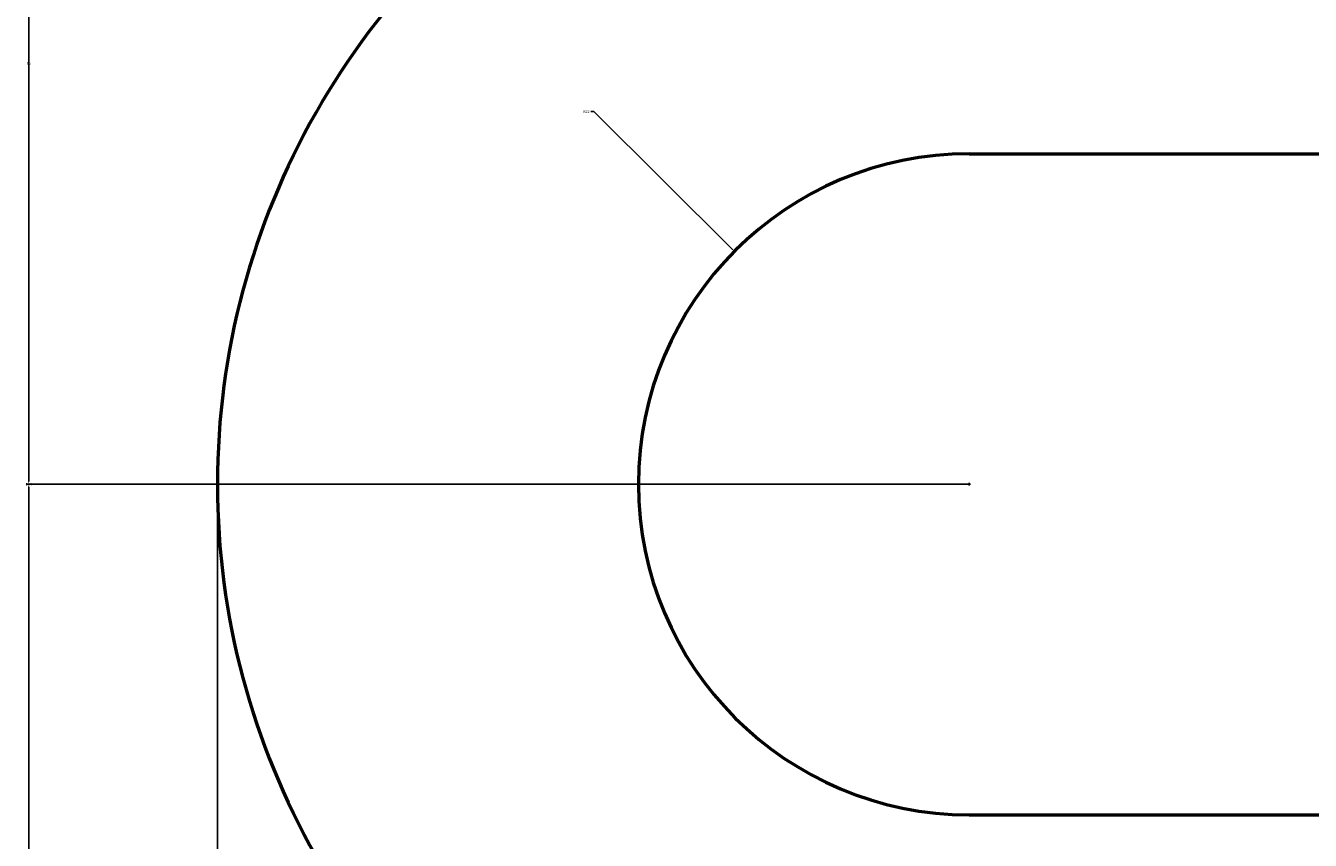
# Model space of a CAD drawing. Units: inches. Extents: x -307 to -76, y 16 to 196.
# Tile 2 of 7: x -307 to -222, y 77 to 132. Entities that reach past the tile are written whole.
import ezdxf

# ---------------------------------------------------------------- set-up
doc = ezdxf.new("R2010")
doc.units = ezdxf.units.IN
doc.header["$MEASUREMENT"] = 0
doc.layers.add('M-DIMS', color=2, linetype='Continuous', lineweight=18)
doc.layers.add('M-OUTL', color=7, linetype='Continuous', lineweight=50)
doc.styles.get("Standard").update_dxf_attribs({"font": 'arial.ttf'})
doc.dimstyles.get("Standard").update_dxf_attribs({"dimtxt": 0.18, "dimasz": 0.18, "dimexe": 0.18, "dimexo": 0.0625, "dimgap": 0.09, "dimtad": 0, "dimtih": 1, "dimtoh": 1, "dimdec": 4, "dimzin": 0, "dimdsep": 46, "dimtxsty": 'Standard', "dimcen": 0.09, "dimadec": 0, "dimazin": 0, "dimtfac": 1, "dimtdec": 4, "dimtofl": 0, "dimtmove": 0, "dimatfit": 3, "dimfxl": 1, "dimtolj": 1, "dimtzin": 0, "dimarcsym": 0})

# ---------------------------------------------------------------- blocks, each defined once
blk = doc.blocks.new('*D2')
at = {"layer": 'Defpoints', "color": 0, "transparency": 16777216}
for p in [(-294.39, 101), (-88.39, 101), (-88.39, 16.45)]:
    blk.add_point(p, dxfattribs=at)
at = {"layer": 'M-DIMS', "color": 0, "lineweight": -2, "transparency": 16777216}
for p, q in [((-294.39, 100.938), (-294.39, 16.27)), ((-88.39, 100.938), (-88.39, 16.27)), ((-294.21, 16.45), (-191.68, 16.45)), ((-88.57, 16.45), (-191.099, 16.45))]:
    blk.add_line(p, q, dxfattribs=at)
at = {"layer": 'M-DIMS', "color": 0, "transparency": 16777216}
for points in [[(-294.21, 16.48), (-294.21, 16.42), (-294.39, 16.45)], [(-88.57, 16.48), (-88.57, 16.42), (-88.39, 16.45)]]:
    blk.add_solid(points, dxfattribs=at)
at = {"layer": 'M-DIMS', "color": 0, "transparency": 16777216, "insert": (-191.39, 16.45), "char_height": 0.18, "attachment_point": 5}
blk.add_mtext('\\A1;206', dxfattribs=at)
blk = doc.blocks.new('*D3')
at = {"layer": 'Defpoints', "color": 0, "transparency": 16777216}
for p in [(-306.94, 173), (-244.39, 173), (-244.39, 29)]:
    blk.add_point(p, dxfattribs=at)
at = {"layer": 'M-DIMS', "color": 0, "lineweight": -2, "transparency": 16777216}
for p, q in [((-244.452, 173), (-307.12, 173)), ((-306.94, 172.82), (-306.94, 101.18)), ((-306.94, 29.18), (-306.94, 100.82)), ((-244.452, 29), (-307.12, 29))]:
    blk.add_line(p, q, dxfattribs=at)
at = {"layer": 'M-DIMS', "color": 0, "transparency": 16777216}
for points in [[(-306.97, 172.82), (-306.91, 172.82), (-306.94, 173)], [(-306.97, 29.18), (-306.91, 29.18), (-306.94, 29)]]:
    blk.add_solid(points, dxfattribs=at)
at = {"layer": 'M-DIMS', "color": 0, "transparency": 16777216, "insert": (-306.94, 101), "char_height": 0.18, "attachment_point": 5}
blk.add_mtext('\\A1;144', dxfattribs=at)
blk = doc.blocks.new('*D4')
at = {"layer": 'Defpoints', "color": 0, "transparency": 16777216}
for p in [(-203.39, 185.55), (-244.39, 157), (-203.39, 101)]:
    blk.add_point(p, dxfattribs=at)
at = {"layer": 'M-DIMS', "color": 0, "lineweight": -2, "transparency": 16777216}
for p, q in [((-244.39, 157.062), (-244.39, 185.73)), ((-244.21, 185.55), (-224.095, 185.55)), ((-203.57, 185.55), (-223.684, 185.55)), ((-203.39, 101.062), (-203.39, 185.73))]:
    blk.add_line(p, q, dxfattribs=at)
at = {"layer": 'M-DIMS', "color": 0, "transparency": 16777216}
for points in [[(-244.21, 185.58), (-244.21, 185.52), (-244.39, 185.55)], [(-203.57, 185.58), (-203.57, 185.52), (-203.39, 185.55)]]:
    blk.add_solid(points, dxfattribs=at)
at = {"layer": 'M-DIMS', "color": 0, "transparency": 16777216, "insert": (-223.89, 185.55), "char_height": 0.18, "attachment_point": 5}
blk.add_mtext('\\A1;41', dxfattribs=at)
blk = doc.blocks.new('*D6')
at = {"layer": 'Defpoints', "color": 0, "transparency": 16777216}
for p in [(-306.94, 101), (-244.39, 101), (-244.39, 45)]:
    blk.add_point(p, dxfattribs=at)
at = {"layer": 'M-DIMS', "color": 0, "lineweight": -2, "transparency": 16777216}
for p, q in [((-244.452, 101), (-307.12, 101)), ((-306.94, 100.82), (-306.94, 73.182)), ((-306.94, 45.18), (-306.94, 72.818)), ((-244.452, 45), (-307.12, 45))]:
    blk.add_line(p, q, dxfattribs=at)
at = {"layer": 'M-DIMS', "color": 0, "transparency": 16777216}
for points in [[(-306.97, 100.82), (-306.91, 100.82), (-306.94, 101)], [(-306.97, 45.18), (-306.91, 45.18), (-306.94, 45)]]:
    blk.add_solid(points, dxfattribs=at)
at = {"layer": 'M-DIMS', "color": 0, "transparency": 16777216, "insert": (-306.94, 73), "char_height": 0.18, "attachment_point": 5}
blk.add_mtext('\\A1;56', dxfattribs=at)
blk = doc.blocks.new('*D7')
at = {"layer": 'Defpoints', "color": 0, "transparency": 16777216}
for p in [(-306.94, 157), (-244.39, 157), (-244.39, 101)]:
    blk.add_point(p, dxfattribs=at)
at = {"layer": 'M-DIMS', "color": 0, "lineweight": -2, "transparency": 16777216}
for p, q in [((-244.452, 157), (-307.12, 157)), ((-306.94, 156.82), (-306.94, 129.182)), ((-306.94, 101.18), (-306.94, 128.818)), ((-244.452, 101), (-307.12, 101))]:
    blk.add_line(p, q, dxfattribs=at)
at = {"layer": 'M-DIMS', "color": 0, "transparency": 16777216}
for points in [[(-306.97, 156.82), (-306.91, 156.82), (-306.94, 157)], [(-306.97, 101.18), (-306.91, 101.18), (-306.94, 101)]]:
    blk.add_solid(points, dxfattribs=at)
at = {"layer": 'M-DIMS', "color": 0, "transparency": 16777216, "insert": (-306.94, 129), "char_height": 0.18, "attachment_point": 5}
blk.add_mtext('\\A1;56', dxfattribs=at)
blk = doc.blocks.new('*D12')
at = {"layer": 'Defpoints', "color": 0, "transparency": 16777216}
for p in [(-260.001, 116.501), (-244.39, 101)]:
    blk.add_point(p, dxfattribs=at)
at = {"layer": 'M-DIMS', "color": 0, "lineweight": -2, "transparency": 16777216}
for p, q in [((-269.548, 125.802), (-269.368, 125.802)), ((-269.368, 125.802), (-260.129, 116.628)), ((-244.48, 101), (-244.3, 101)), ((-244.39, 100.91), (-244.39, 101.09))]:
    blk.add_line(p, q, dxfattribs=at)
at = {"layer": 'M-DIMS', "color": 0, "transparency": 16777216}
blk.add_solid([(-260.108, 116.649), (-260.15, 116.607), (-260.001, 116.501)], dxfattribs=at)
at = {"layer": 'M-DIMS', "color": 0, "transparency": 16777216, "insert": (-269.852, 125.802), "char_height": 0.18, "attachment_point": 5}
blk.add_mtext('\\A1;R22', dxfattribs=at)

msp = doc.modelspace()

# ---------------------------------------------------------------- linework, layer by layer
at = {"layer": 'M-OUTL'}
for p, q in [((-244.39, 123), (-159.193, 123)), ((-244.39, 79), (-159.518, 79))]:
    msp.add_line(p, q, dxfattribs=at)
for radius, start, end in [(50, 120.71777, 239.28223), (22, 90, 270)]:
    msp.add_arc((-244.39, 101), radius, start, end, dxfattribs=at)

# ---------------------------------------------------------------- dimensions: what is measured, and where the dimension line sits
at = {"layer": 'M-DIMS'}
for base, p1, p2, picture, middle in [((-203.39, 185.55), (-244.39, 157), (-203.39, 101), '*D4', (-223.89, 185.55)), ((-88.39, 16.45), (-294.39, 101), (-88.39, 101), '*D2', (-191.39, 16.45))]:
    dim = msp.add_linear_dim(base=base, p1=p1, p2=p2, dimstyle='Standard', override={"dimdec": 0, "dimlfac": 1, "dimrnd": 0, "dimzin": 0, "dimdsep": 46, "dimlunit": 2}, dxfattribs=at)
    dim.commit()
    dim.dimension.update_dxf_attribs({"geometry": picture, "text_midpoint": middle})
for base, p1, p2, picture, middle in [((-306.94, 173), (-244.39, 29), (-244.39, 173), '*D3', (-306.94, 101)), ((-306.94, 157), (-244.39, 101), (-244.39, 157), '*D7', (-306.94, 129)), ((-306.94, 101), (-244.39, 45), (-244.39, 101), '*D6', (-306.94, 73))]:
    dim = msp.add_linear_dim(base=base, p1=p1, p2=p2, angle=90, dimstyle='Standard', override={"dimdec": 0, "dimlfac": 1, "dimrnd": 0, "dimzin": 0, "dimdsep": 46, "dimlunit": 2}, dxfattribs=at)
    dim.commit()
    dim.dimension.update_dxf_attribs({"geometry": picture, "text_midpoint": middle})
dim = msp.add_radius_dim(center=(-244.39, 101), mpoint=(-260.001, 116.501), dimstyle='Standard', override={"dimdec": 0, "dimlfac": 1, "dimrnd": 0, "dimzin": 0, "dimdsep": 46, "dimlunit": 2}, dxfattribs=at)
dim.commit()
dim.dimension.update_dxf_attribs({"geometry": '*D12', "text_midpoint": (-269.852, 125.802), "dimtype": 164})

doc.saveas('drawing.dxf')
